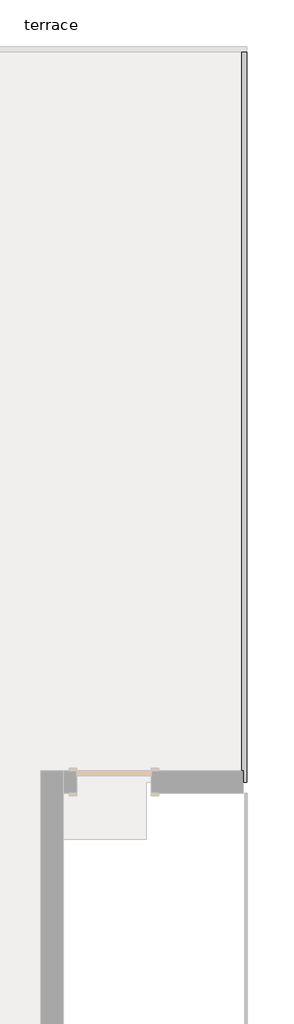
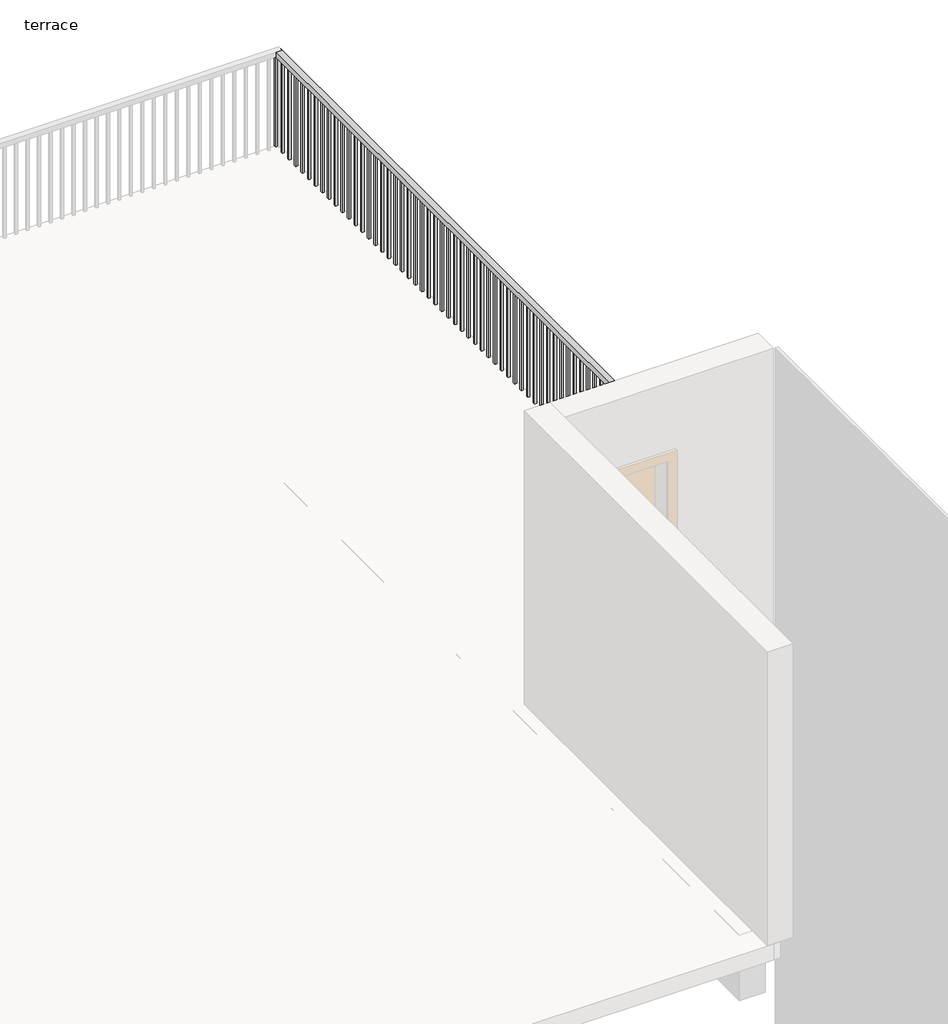
# One storey, part 6 of 6: 1 railing.
"""IFC4 building model written with IfcOpenShell, lengths in millimetres."""

from ifc_helpers import new_model, si_unit, frame, origin, place, context, project, spatial, polyline, outline, extrude, element, save

model = new_model("IFC4")

# Units and contexts
model_context = context("Model", 3, world=origin())
ifc_project = project(units=[si_unit("LENGTHUNIT", "METRE", prefix="MILLI")], contexts=[model_context])

# Site, building, storey
site = spatial("IfcSite", under=ifc_project)
building = spatial("IfcBuilding", under=site)
storey = spatial("IfcBuildingStorey", under=building, Name="terrace", Elevation=7010.4)

# Railing
placement = place(None, origin())
element("IfcRailing", 1, ObjectType="Handrail - Rectangular", at=placement, inside=storey, context=model_context, shape_type="SweptSolid", body=[
    extrude(outline(polyline([(-2647.3594779, -998.5064015), (-2698.1594779, -998.5064015), (-2698.1594779, 6526.2435985), (-2647.3594779, 6526.2435985), (-2647.3594779, -998.5064015)])), frame((0.0, 0.0, 7874.0), z_axis=(0.0, 0.0, 1.0), x_axis=(1.0, 0.0, 0.0)), (0.0, 0.0, 1.0), 50.8),
    extrude(outline(polyline([(-2663.2344779, 6510.3685985), (-2682.2844779, 6510.3685985), (-2682.2844779, 6529.4185985), (-2663.2344779, 6529.4185985), (-2663.2344779, 6510.3685985)])), frame((0.0, 0.0, 7010.4), z_axis=(0.0, 0.0, 1.0), x_axis=(1.0, 0.0, 0.0)), (0.0, 0.0, 1.0), 863.6),
    extrude(outline(polyline([(-2663.2344779, 6408.7685985), (-2682.2844779, 6408.7685985), (-2682.2844779, 6427.8185985), (-2663.2344779, 6427.8185985), (-2663.2344779, 6408.7685985)])), frame((0.0, 0.0, 7010.4), z_axis=(0.0, 0.0, 1.0), x_axis=(1.0, 0.0, 0.0)), (0.0, 0.0, 1.0), 863.6),
    extrude(outline(polyline([(-2663.2344779, 6307.1685985), (-2682.2844779, 6307.1685985), (-2682.2844779, 6326.2185985), (-2663.2344779, 6326.2185985), (-2663.2344779, 6307.1685985)])), frame((0.0, 0.0, 7010.4), z_axis=(0.0, 0.0, 1.0), x_axis=(1.0, 0.0, 0.0)), (0.0, 0.0, 1.0), 863.6),
    extrude(outline(polyline([(-2663.2344779, 6205.5685985), (-2682.2844779, 6205.5685985), (-2682.2844779, 6224.6185985), (-2663.2344779, 6224.6185985), (-2663.2344779, 6205.5685985)])), frame((0.0, 0.0, 7010.4), z_axis=(0.0, 0.0, 1.0), x_axis=(1.0, 0.0, 0.0)), (0.0, 0.0, 1.0), 863.6),
    extrude(outline(polyline([(-2663.2344779, 6103.9685985), (-2682.2844779, 6103.9685985), (-2682.2844779, 6123.0185985), (-2663.2344779, 6123.0185985), (-2663.2344779, 6103.9685985)])), frame((0.0, 0.0, 7010.4), z_axis=(0.0, 0.0, 1.0), x_axis=(1.0, 0.0, 0.0)), (0.0, 0.0, 1.0), 863.6),
    extrude(outline(polyline([(-2663.2344779, 6002.3685985), (-2682.2844779, 6002.3685985), (-2682.2844779, 6021.4185985), (-2663.2344779, 6021.4185985), (-2663.2344779, 6002.3685985)])), frame((0.0, 0.0, 7010.4), z_axis=(0.0, 0.0, 1.0), x_axis=(1.0, 0.0, 0.0)), (0.0, 0.0, 1.0), 863.6),
    extrude(outline(polyline([(-2663.2344779, 5900.7685985), (-2682.2844779, 5900.7685985), (-2682.2844779, 5919.8185985), (-2663.2344779, 5919.8185985), (-2663.2344779, 5900.7685985)])), frame((0.0, 0.0, 7010.4), z_axis=(0.0, 0.0, 1.0), x_axis=(1.0, 0.0, 0.0)), (0.0, 0.0, 1.0), 863.6),
    extrude(outline(polyline([(-2663.2344779, 5799.1685985), (-2682.2844779, 5799.1685985), (-2682.2844779, 5818.2185985), (-2663.2344779, 5818.2185985), (-2663.2344779, 5799.1685985)])), frame((0.0, 0.0, 7010.4), z_axis=(0.0, 0.0, 1.0), x_axis=(1.0, 0.0, 0.0)), (0.0, 0.0, 1.0), 863.6),
    extrude(outline(polyline([(-2663.2344779, 5697.5685985), (-2682.2844779, 5697.5685985), (-2682.2844779, 5716.6185985), (-2663.2344779, 5716.6185985), (-2663.2344779, 5697.5685985)])), frame((0.0, 0.0, 7010.4), z_axis=(0.0, 0.0, 1.0), x_axis=(1.0, 0.0, 0.0)), (0.0, 0.0, 1.0), 863.6),
    extrude(outline(polyline([(-2663.2344779, 5595.9685985), (-2682.2844779, 5595.9685985), (-2682.2844779, 5615.0185985), (-2663.2344779, 5615.0185985), (-2663.2344779, 5595.9685985)])), frame((0.0, 0.0, 7010.4), z_axis=(0.0, 0.0, 1.0), x_axis=(1.0, 0.0, 0.0)), (0.0, 0.0, 1.0), 863.6),
    extrude(outline(polyline([(-2663.2344779, 5494.3685985), (-2682.2844779, 5494.3685985), (-2682.2844779, 5513.4185985), (-2663.2344779, 5513.4185985), (-2663.2344779, 5494.3685985)])), frame((0.0, 0.0, 7010.4), z_axis=(0.0, 0.0, 1.0), x_axis=(1.0, 0.0, 0.0)), (0.0, 0.0, 1.0), 863.6),
    extrude(outline(polyline([(-2663.2344779, 5392.7685985), (-2682.2844779, 5392.7685985), (-2682.2844779, 5411.8185985), (-2663.2344779, 5411.8185985), (-2663.2344779, 5392.7685985)])), frame((0.0, 0.0, 7010.4), z_axis=(0.0, 0.0, 1.0), x_axis=(1.0, 0.0, 0.0)), (0.0, 0.0, 1.0), 863.6),
    extrude(outline(polyline([(-2663.2344779, 5291.1685985), (-2682.2844779, 5291.1685985), (-2682.2844779, 5310.2185985), (-2663.2344779, 5310.2185985), (-2663.2344779, 5291.1685985)])), frame((0.0, 0.0, 7010.4), z_axis=(0.0, 0.0, 1.0), x_axis=(1.0, 0.0, 0.0)), (0.0, 0.0, 1.0), 863.6),
    extrude(outline(polyline([(-2663.2344779, 5189.5685985), (-2682.2844779, 5189.5685985), (-2682.2844779, 5208.6185985), (-2663.2344779, 5208.6185985), (-2663.2344779, 5189.5685985)])), frame((0.0, 0.0, 7010.4), z_axis=(0.0, 0.0, 1.0), x_axis=(1.0, 0.0, 0.0)), (0.0, 0.0, 1.0), 863.6),
    extrude(outline(polyline([(-2663.2344779, 5087.9685985), (-2682.2844779, 5087.9685985), (-2682.2844779, 5107.0185985), (-2663.2344779, 5107.0185985), (-2663.2344779, 5087.9685985)])), frame((0.0, 0.0, 7010.4), z_axis=(0.0, 0.0, 1.0), x_axis=(1.0, 0.0, 0.0)), (0.0, 0.0, 1.0), 863.6),
    extrude(outline(polyline([(-2663.2344779, 4986.3685985), (-2682.2844779, 4986.3685985), (-2682.2844779, 5005.4185985), (-2663.2344779, 5005.4185985), (-2663.2344779, 4986.3685985)])), frame((0.0, 0.0, 7010.4), z_axis=(0.0, 0.0, 1.0), x_axis=(1.0, 0.0, 0.0)), (0.0, 0.0, 1.0), 863.6),
    extrude(outline(polyline([(-2663.2344779, 4884.7685985), (-2682.2844779, 4884.7685985), (-2682.2844779, 4903.8185985), (-2663.2344779, 4903.8185985), (-2663.2344779, 4884.7685985)])), frame((0.0, 0.0, 7010.4), z_axis=(0.0, 0.0, 1.0), x_axis=(1.0, 0.0, 0.0)), (0.0, 0.0, 1.0), 863.6),
    extrude(outline(polyline([(-2663.2344779, 4783.1685985), (-2682.2844779, 4783.1685985), (-2682.2844779, 4802.2185985), (-2663.2344779, 4802.2185985), (-2663.2344779, 4783.1685985)])), frame((0.0, 0.0, 7010.4), z_axis=(0.0, 0.0, 1.0), x_axis=(1.0, 0.0, 0.0)), (0.0, 0.0, 1.0), 863.6),
    extrude(outline(polyline([(-2663.2344779, 4681.5685985), (-2682.2844779, 4681.5685985), (-2682.2844779, 4700.6185985), (-2663.2344779, 4700.6185985), (-2663.2344779, 4681.5685985)])), frame((0.0, 0.0, 7010.4), z_axis=(0.0, 0.0, 1.0), x_axis=(1.0, 0.0, 0.0)), (0.0, 0.0, 1.0), 863.6),
    extrude(outline(polyline([(-2663.2344779, 4579.9685985), (-2682.2844779, 4579.9685985), (-2682.2844779, 4599.0185985), (-2663.2344779, 4599.0185985), (-2663.2344779, 4579.9685985)])), frame((0.0, 0.0, 7010.4), z_axis=(0.0, 0.0, 1.0), x_axis=(1.0, 0.0, 0.0)), (0.0, 0.0, 1.0), 863.6),
    extrude(outline(polyline([(-2663.2344779, 4478.3685985), (-2682.2844779, 4478.3685985), (-2682.2844779, 4497.4185985), (-2663.2344779, 4497.4185985), (-2663.2344779, 4478.3685985)])), frame((0.0, 0.0, 7010.4), z_axis=(0.0, 0.0, 1.0), x_axis=(1.0, 0.0, 0.0)), (0.0, 0.0, 1.0), 863.6),
    extrude(outline(polyline([(-2663.2344779, 4376.7685985), (-2682.2844779, 4376.7685985), (-2682.2844779, 4395.8185985), (-2663.2344779, 4395.8185985), (-2663.2344779, 4376.7685985)])), frame((0.0, 0.0, 7010.4), z_axis=(0.0, 0.0, 1.0), x_axis=(1.0, 0.0, 0.0)), (0.0, 0.0, 1.0), 863.6),
    extrude(outline(polyline([(-2663.2344779, 4275.1685985), (-2682.2844779, 4275.1685985), (-2682.2844779, 4294.2185985), (-2663.2344779, 4294.2185985), (-2663.2344779, 4275.1685985)])), frame((0.0, 0.0, 7010.4), z_axis=(0.0, 0.0, 1.0), x_axis=(1.0, 0.0, 0.0)), (0.0, 0.0, 1.0), 863.6),
    extrude(outline(polyline([(-2663.2344779, 4173.5685985), (-2682.2844779, 4173.5685985), (-2682.2844779, 4192.6185985), (-2663.2344779, 4192.6185985), (-2663.2344779, 4173.5685985)])), frame((0.0, 0.0, 7010.4), z_axis=(0.0, 0.0, 1.0), x_axis=(1.0, 0.0, 0.0)), (0.0, 0.0, 1.0), 863.6),
    extrude(outline(polyline([(-2663.2344779, 4071.9685985), (-2682.2844779, 4071.9685985), (-2682.2844779, 4091.0185985), (-2663.2344779, 4091.0185985), (-2663.2344779, 4071.9685985)])), frame((0.0, 0.0, 7010.4), z_axis=(0.0, 0.0, 1.0), x_axis=(1.0, 0.0, 0.0)), (0.0, 0.0, 1.0), 863.6),
    extrude(outline(polyline([(-2663.2344779, 3970.3685985), (-2682.2844779, 3970.3685985), (-2682.2844779, 3989.4185985), (-2663.2344779, 3989.4185985), (-2663.2344779, 3970.3685985)])), frame((0.0, 0.0, 7010.4), z_axis=(0.0, 0.0, 1.0), x_axis=(1.0, 0.0, 0.0)), (0.0, 0.0, 1.0), 863.6),
    extrude(outline(polyline([(-2663.2344779, 3868.7685985), (-2682.2844779, 3868.7685985), (-2682.2844779, 3887.8185985), (-2663.2344779, 3887.8185985), (-2663.2344779, 3868.7685985)])), frame((0.0, 0.0, 7010.4), z_axis=(0.0, 0.0, 1.0), x_axis=(1.0, 0.0, 0.0)), (0.0, 0.0, 1.0), 863.6),
    extrude(outline(polyline([(-2663.2344779, 3767.1685985), (-2682.2844779, 3767.1685985), (-2682.2844779, 3786.2185985), (-2663.2344779, 3786.2185985), (-2663.2344779, 3767.1685985)])), frame((0.0, 0.0, 7010.4), z_axis=(0.0, 0.0, 1.0), x_axis=(1.0, 0.0, 0.0)), (0.0, 0.0, 1.0), 863.6),
    extrude(outline(polyline([(-2663.2344779, 3665.5685985), (-2682.2844779, 3665.5685985), (-2682.2844779, 3684.6185985), (-2663.2344779, 3684.6185985), (-2663.2344779, 3665.5685985)])), frame((0.0, 0.0, 7010.4), z_axis=(0.0, 0.0, 1.0), x_axis=(1.0, 0.0, 0.0)), (0.0, 0.0, 1.0), 863.6),
    extrude(outline(polyline([(-2663.2344779, 3563.9685985), (-2682.2844779, 3563.9685985), (-2682.2844779, 3583.0185985), (-2663.2344779, 3583.0185985), (-2663.2344779, 3563.9685985)])), frame((0.0, 0.0, 7010.4), z_axis=(0.0, 0.0, 1.0), x_axis=(1.0, 0.0, 0.0)), (0.0, 0.0, 1.0), 863.6),
    extrude(outline(polyline([(-2663.2344779, 3462.3685985), (-2682.2844779, 3462.3685985), (-2682.2844779, 3481.4185985), (-2663.2344779, 3481.4185985), (-2663.2344779, 3462.3685985)])), frame((0.0, 0.0, 7010.4), z_axis=(0.0, 0.0, 1.0), x_axis=(1.0, 0.0, 0.0)), (0.0, 0.0, 1.0), 863.6),
    extrude(outline(polyline([(-2663.2344779, 3360.7685985), (-2682.2844779, 3360.7685985), (-2682.2844779, 3379.8185985), (-2663.2344779, 3379.8185985), (-2663.2344779, 3360.7685985)])), frame((0.0, 0.0, 7010.4), z_axis=(0.0, 0.0, 1.0), x_axis=(1.0, 0.0, 0.0)), (0.0, 0.0, 1.0), 863.6),
    extrude(outline(polyline([(-2663.2344779, 3259.1685985), (-2682.2844779, 3259.1685985), (-2682.2844779, 3278.2185985), (-2663.2344779, 3278.2185985), (-2663.2344779, 3259.1685985)])), frame((0.0, 0.0, 7010.4), z_axis=(0.0, 0.0, 1.0), x_axis=(1.0, 0.0, 0.0)), (0.0, 0.0, 1.0), 863.6),
    extrude(outline(polyline([(-2663.2344779, 3157.5685985), (-2682.2844779, 3157.5685985), (-2682.2844779, 3176.6185985), (-2663.2344779, 3176.6185985), (-2663.2344779, 3157.5685985)])), frame((0.0, 0.0, 7010.4), z_axis=(0.0, 0.0, 1.0), x_axis=(1.0, 0.0, 0.0)), (0.0, 0.0, 1.0), 863.6),
    extrude(outline(polyline([(-2663.2344779, 3055.9685985), (-2682.2844779, 3055.9685985), (-2682.2844779, 3075.0185985), (-2663.2344779, 3075.0185985), (-2663.2344779, 3055.9685985)])), frame((0.0, 0.0, 7010.4), z_axis=(0.0, 0.0, 1.0), x_axis=(1.0, 0.0, 0.0)), (0.0, 0.0, 1.0), 863.6),
    extrude(outline(polyline([(-2663.2344779, 2954.3685985), (-2682.2844779, 2954.3685985), (-2682.2844779, 2973.4185985), (-2663.2344779, 2973.4185985), (-2663.2344779, 2954.3685985)])), frame((0.0, 0.0, 7010.4), z_axis=(0.0, 0.0, 1.0), x_axis=(1.0, 0.0, 0.0)), (0.0, 0.0, 1.0), 863.6),
    extrude(outline(polyline([(-2663.2344779, 2852.7685985), (-2682.2844779, 2852.7685985), (-2682.2844779, 2871.8185985), (-2663.2344779, 2871.8185985), (-2663.2344779, 2852.7685985)])), frame((0.0, 0.0, 7010.4), z_axis=(0.0, 0.0, 1.0), x_axis=(1.0, 0.0, 0.0)), (0.0, 0.0, 1.0), 863.6),
    extrude(outline(polyline([(-2663.2344779, 2751.1685985), (-2682.2844779, 2751.1685985), (-2682.2844779, 2770.2185985), (-2663.2344779, 2770.2185985), (-2663.2344779, 2751.1685985)])), frame((0.0, 0.0, 7010.4), z_axis=(0.0, 0.0, 1.0), x_axis=(1.0, 0.0, 0.0)), (0.0, 0.0, 1.0), 863.6),
    extrude(outline(polyline([(-2663.2344779, 2649.5685985), (-2682.2844779, 2649.5685985), (-2682.2844779, 2668.6185985), (-2663.2344779, 2668.6185985), (-2663.2344779, 2649.5685985)])), frame((0.0, 0.0, 7010.4), z_axis=(0.0, 0.0, 1.0), x_axis=(1.0, 0.0, 0.0)), (0.0, 0.0, 1.0), 863.6),
    extrude(outline(polyline([(-2663.2344779, 2547.9685985), (-2682.2844779, 2547.9685985), (-2682.2844779, 2567.0185985), (-2663.2344779, 2567.0185985), (-2663.2344779, 2547.9685985)])), frame((0.0, 0.0, 7010.4), z_axis=(0.0, 0.0, 1.0), x_axis=(1.0, 0.0, 0.0)), (0.0, 0.0, 1.0), 863.6),
    extrude(outline(polyline([(-2663.2344779, 2446.3685985), (-2682.2844779, 2446.3685985), (-2682.2844779, 2465.4185985), (-2663.2344779, 2465.4185985), (-2663.2344779, 2446.3685985)])), frame((0.0, 0.0, 7010.4), z_axis=(0.0, 0.0, 1.0), x_axis=(1.0, 0.0, 0.0)), (0.0, 0.0, 1.0), 863.6),
    extrude(outline(polyline([(-2663.2344779, 2344.7685985), (-2682.2844779, 2344.7685985), (-2682.2844779, 2363.8185985), (-2663.2344779, 2363.8185985), (-2663.2344779, 2344.7685985)])), frame((0.0, 0.0, 7010.4), z_axis=(0.0, 0.0, 1.0), x_axis=(1.0, 0.0, 0.0)), (0.0, 0.0, 1.0), 863.6),
    extrude(outline(polyline([(-2663.2344779, 2243.1685985), (-2682.2844779, 2243.1685985), (-2682.2844779, 2262.2185985), (-2663.2344779, 2262.2185985), (-2663.2344779, 2243.1685985)])), frame((0.0, 0.0, 7010.4), z_axis=(0.0, 0.0, 1.0), x_axis=(1.0, 0.0, 0.0)), (0.0, 0.0, 1.0), 863.6),
    extrude(outline(polyline([(-2663.2344779, 2141.5685985), (-2682.2844779, 2141.5685985), (-2682.2844779, 2160.6185985), (-2663.2344779, 2160.6185985), (-2663.2344779, 2141.5685985)])), frame((0.0, 0.0, 7010.4), z_axis=(0.0, 0.0, 1.0), x_axis=(1.0, 0.0, 0.0)), (0.0, 0.0, 1.0), 863.6),
    extrude(outline(polyline([(-2663.2344779, 2039.9685985), (-2682.2844779, 2039.9685985), (-2682.2844779, 2059.0185985), (-2663.2344779, 2059.0185985), (-2663.2344779, 2039.9685985)])), frame((0.0, 0.0, 7010.4), z_axis=(0.0, 0.0, 1.0), x_axis=(1.0, 0.0, 0.0)), (0.0, 0.0, 1.0), 863.6),
    extrude(outline(polyline([(-2663.2344779, 1938.3685985), (-2682.2844779, 1938.3685985), (-2682.2844779, 1957.4185985), (-2663.2344779, 1957.4185985), (-2663.2344779, 1938.3685985)])), frame((0.0, 0.0, 7010.4), z_axis=(0.0, 0.0, 1.0), x_axis=(1.0, 0.0, 0.0)), (0.0, 0.0, 1.0), 863.6),
    extrude(outline(polyline([(-2663.2344779, 1836.7685985), (-2682.2844779, 1836.7685985), (-2682.2844779, 1855.8185985), (-2663.2344779, 1855.8185985), (-2663.2344779, 1836.7685985)])), frame((0.0, 0.0, 7010.4), z_axis=(0.0, 0.0, 1.0), x_axis=(1.0, 0.0, 0.0)), (0.0, 0.0, 1.0), 863.6),
    extrude(outline(polyline([(-2663.2344779, 1735.1685985), (-2682.2844779, 1735.1685985), (-2682.2844779, 1754.2185985), (-2663.2344779, 1754.2185985), (-2663.2344779, 1735.1685985)])), frame((0.0, 0.0, 7010.4), z_axis=(0.0, 0.0, 1.0), x_axis=(1.0, 0.0, 0.0)), (0.0, 0.0, 1.0), 863.6),
    extrude(outline(polyline([(-2663.2344779, 1633.5685985), (-2682.2844779, 1633.5685985), (-2682.2844779, 1652.6185985), (-2663.2344779, 1652.6185985), (-2663.2344779, 1633.5685985)])), frame((0.0, 0.0, 7010.4), z_axis=(0.0, 0.0, 1.0), x_axis=(1.0, 0.0, 0.0)), (0.0, 0.0, 1.0), 863.6),
    extrude(outline(polyline([(-2663.2344779, 1531.9685985), (-2682.2844779, 1531.9685985), (-2682.2844779, 1551.0185985), (-2663.2344779, 1551.0185985), (-2663.2344779, 1531.9685985)])), frame((0.0, 0.0, 7010.4), z_axis=(0.0, 0.0, 1.0), x_axis=(1.0, 0.0, 0.0)), (0.0, 0.0, 1.0), 863.6),
    extrude(outline(polyline([(-2663.2344779, 1430.3685985), (-2682.2844779, 1430.3685985), (-2682.2844779, 1449.4185985), (-2663.2344779, 1449.4185985), (-2663.2344779, 1430.3685985)])), frame((0.0, 0.0, 7010.4), z_axis=(0.0, 0.0, 1.0), x_axis=(1.0, 0.0, 0.0)), (0.0, 0.0, 1.0), 863.6),
    extrude(outline(polyline([(-2663.2344779, 1328.7685985), (-2682.2844779, 1328.7685985), (-2682.2844779, 1347.8185985), (-2663.2344779, 1347.8185985), (-2663.2344779, 1328.7685985)])), frame((0.0, 0.0, 7010.4), z_axis=(0.0, 0.0, 1.0), x_axis=(1.0, 0.0, 0.0)), (0.0, 0.0, 1.0), 863.6),
    extrude(outline(polyline([(-2663.2344779, 1227.1685985), (-2682.2844779, 1227.1685985), (-2682.2844779, 1246.2185985), (-2663.2344779, 1246.2185985), (-2663.2344779, 1227.1685985)])), frame((0.0, 0.0, 7010.4), z_axis=(0.0, 0.0, 1.0), x_axis=(1.0, 0.0, 0.0)), (0.0, 0.0, 1.0), 863.6),
    extrude(outline(polyline([(-2663.2344779, 1125.5685985), (-2682.2844779, 1125.5685985), (-2682.2844779, 1144.6185985), (-2663.2344779, 1144.6185985), (-2663.2344779, 1125.5685985)])), frame((0.0, 0.0, 7010.4), z_axis=(0.0, 0.0, 1.0), x_axis=(1.0, 0.0, 0.0)), (0.0, 0.0, 1.0), 863.6),
    extrude(outline(polyline([(-2663.2344779, 1023.9685985), (-2682.2844779, 1023.9685985), (-2682.2844779, 1043.0185985), (-2663.2344779, 1043.0185985), (-2663.2344779, 1023.9685985)])), frame((0.0, 0.0, 7010.4), z_axis=(0.0, 0.0, 1.0), x_axis=(1.0, 0.0, 0.0)), (0.0, 0.0, 1.0), 863.6),
    extrude(outline(polyline([(-2663.2344779, 922.3685985), (-2682.2844779, 922.3685985), (-2682.2844779, 941.4185985), (-2663.2344779, 941.4185985), (-2663.2344779, 922.3685985)])), frame((0.0, 0.0, 7010.4), z_axis=(0.0, 0.0, 1.0), x_axis=(1.0, 0.0, 0.0)), (0.0, 0.0, 1.0), 863.6),
    extrude(outline(polyline([(-2663.2344779, 820.7685985), (-2682.2844779, 820.7685985), (-2682.2844779, 839.8185985), (-2663.2344779, 839.8185985), (-2663.2344779, 820.7685985)])), frame((0.0, 0.0, 7010.4), z_axis=(0.0, 0.0, 1.0), x_axis=(1.0, 0.0, 0.0)), (0.0, 0.0, 1.0), 863.6),
    extrude(outline(polyline([(-2663.2344779, 719.1685985), (-2682.2844779, 719.1685985), (-2682.2844779, 738.2185985), (-2663.2344779, 738.2185985), (-2663.2344779, 719.1685985)])), frame((0.0, 0.0, 7010.4), z_axis=(0.0, 0.0, 1.0), x_axis=(1.0, 0.0, 0.0)), (0.0, 0.0, 1.0), 863.6),
    extrude(outline(polyline([(-2663.2344779, 617.5685985), (-2682.2844779, 617.5685985), (-2682.2844779, 636.6185985), (-2663.2344779, 636.6185985), (-2663.2344779, 617.5685985)])), frame((0.0, 0.0, 7010.4), z_axis=(0.0, 0.0, 1.0), x_axis=(1.0, 0.0, 0.0)), (0.0, 0.0, 1.0), 863.6),
    extrude(outline(polyline([(-2663.2344779, 515.9685985), (-2682.2844779, 515.9685985), (-2682.2844779, 535.0185985), (-2663.2344779, 535.0185985), (-2663.2344779, 515.9685985)])), frame((0.0, 0.0, 7010.4), z_axis=(0.0, 0.0, 1.0), x_axis=(1.0, 0.0, 0.0)), (0.0, 0.0, 1.0), 863.6),
    extrude(outline(polyline([(-2663.2344779, 414.3685985), (-2682.2844779, 414.3685985), (-2682.2844779, 433.4185985), (-2663.2344779, 433.4185985), (-2663.2344779, 414.3685985)])), frame((0.0, 0.0, 7010.4), z_axis=(0.0, 0.0, 1.0), x_axis=(1.0, 0.0, 0.0)), (0.0, 0.0, 1.0), 863.6),
    extrude(outline(polyline([(-2663.2344779, 312.7685985), (-2682.2844779, 312.7685985), (-2682.2844779, 331.8185985), (-2663.2344779, 331.8185985), (-2663.2344779, 312.7685985)])), frame((0.0, 0.0, 7010.4), z_axis=(0.0, 0.0, 1.0), x_axis=(1.0, 0.0, 0.0)), (0.0, 0.0, 1.0), 863.6),
    extrude(outline(polyline([(-2663.2344779, 211.1685985), (-2682.2844779, 211.1685985), (-2682.2844779, 230.2185985), (-2663.2344779, 230.2185985), (-2663.2344779, 211.1685985)])), frame((0.0, 0.0, 7010.4), z_axis=(0.0, 0.0, 1.0), x_axis=(1.0, 0.0, 0.0)), (0.0, 0.0, 1.0), 863.6),
    extrude(outline(polyline([(-2663.2344779, 109.5685985), (-2682.2844779, 109.5685985), (-2682.2844779, 128.6185985), (-2663.2344779, 128.6185985), (-2663.2344779, 109.5685985)])), frame((0.0, 0.0, 7010.4), z_axis=(0.0, 0.0, 1.0), x_axis=(1.0, 0.0, 0.0)), (0.0, 0.0, 1.0), 863.6),
    extrude(outline(polyline([(-2663.2344779, 7.9685985), (-2682.2844779, 7.9685985), (-2682.2844779, 27.0185985), (-2663.2344779, 27.0185985), (-2663.2344779, 7.9685985)])), frame((0.0, 0.0, 7010.4), z_axis=(0.0, 0.0, 1.0), x_axis=(1.0, 0.0, 0.0)), (0.0, 0.0, 1.0), 863.6),
    extrude(outline(polyline([(-2663.2344779, -93.6314015), (-2682.2844779, -93.6314015), (-2682.2844779, -74.5814015), (-2663.2344779, -74.5814015), (-2663.2344779, -93.6314015)])), frame((0.0, 0.0, 7010.4), z_axis=(0.0, 0.0, 1.0), x_axis=(1.0, 0.0, 0.0)), (0.0, 0.0, 1.0), 863.6),
    extrude(outline(polyline([(-2663.2344779, -195.2314015), (-2682.2844779, -195.2314015), (-2682.2844779, -176.1814015), (-2663.2344779, -176.1814015), (-2663.2344779, -195.2314015)])), frame((0.0, 0.0, 7010.4), z_axis=(0.0, 0.0, 1.0), x_axis=(1.0, 0.0, 0.0)), (0.0, 0.0, 1.0), 863.6),
    extrude(outline(polyline([(-2663.2344779, -296.8314015), (-2682.2844779, -296.8314015), (-2682.2844779, -277.7814015), (-2663.2344779, -277.7814015), (-2663.2344779, -296.8314015)])), frame((0.0, 0.0, 7010.4), z_axis=(0.0, 0.0, 1.0), x_axis=(1.0, 0.0, 0.0)), (0.0, 0.0, 1.0), 863.6),
    extrude(outline(polyline([(-2663.2344779, -398.4314015), (-2682.2844779, -398.4314015), (-2682.2844779, -379.3814015), (-2663.2344779, -379.3814015), (-2663.2344779, -398.4314015)])), frame((0.0, 0.0, 7010.4), z_axis=(0.0, 0.0, 1.0), x_axis=(1.0, 0.0, 0.0)), (0.0, 0.0, 1.0), 863.6),
    extrude(outline(polyline([(-2663.2344779, -500.0314015), (-2682.2844779, -500.0314015), (-2682.2844779, -480.9814015), (-2663.2344779, -480.9814015), (-2663.2344779, -500.0314015)])), frame((0.0, 0.0, 7010.4), z_axis=(0.0, 0.0, 1.0), x_axis=(1.0, 0.0, 0.0)), (0.0, 0.0, 1.0), 863.6),
    extrude(outline(polyline([(-2663.2344779, -601.6314015), (-2682.2844779, -601.6314015), (-2682.2844779, -582.5814015), (-2663.2344779, -582.5814015), (-2663.2344779, -601.6314015)])), frame((0.0, 0.0, 7010.4), z_axis=(0.0, 0.0, 1.0), x_axis=(1.0, 0.0, 0.0)), (0.0, 0.0, 1.0), 863.6),
    extrude(outline(polyline([(-2663.2344779, -703.2314015), (-2682.2844779, -703.2314015), (-2682.2844779, -684.1814015), (-2663.2344779, -684.1814015), (-2663.2344779, -703.2314015)])), frame((0.0, 0.0, 7010.4), z_axis=(0.0, 0.0, 1.0), x_axis=(1.0, 0.0, 0.0)), (0.0, 0.0, 1.0), 863.6),
    extrude(outline(polyline([(-2663.2344779, -804.8314015), (-2682.2844779, -804.8314015), (-2682.2844779, -785.7814015), (-2663.2344779, -785.7814015), (-2663.2344779, -804.8314015)])), frame((0.0, 0.0, 7010.4), z_axis=(0.0, 0.0, 1.0), x_axis=(1.0, 0.0, 0.0)), (0.0, 0.0, 1.0), 863.6),
    extrude(outline(polyline([(-2663.2344779, -906.4314015), (-2682.2844779, -906.4314015), (-2682.2844779, -887.3814015), (-2663.2344779, -887.3814015), (-2663.2344779, -906.4314015)])), frame((0.0, 0.0, 7010.4), z_axis=(0.0, 0.0, 1.0), x_axis=(1.0, 0.0, 0.0)), (0.0, 0.0, 1.0), 863.6),
    extrude(outline(polyline([(-2663.2344779, 6507.1935985), (-2682.2844779, 6507.1935985), (-2682.2844779, 6526.2435985), (-2663.2344779, 6526.2435985), (-2663.2344779, 6507.1935985)])), frame((0.0, 0.0, 7010.4), z_axis=(0.0, 0.0, 1.0), x_axis=(1.0, 0.0, 0.0)), (0.0, 0.0, 1.0), 863.6),
    extrude(outline(polyline([(-2663.2344779, -998.5064015), (-2682.2844779, -998.5064015), (-2682.2844779, -979.4564015), (-2663.2344779, -979.4564015), (-2663.2344779, -998.5064015)])), frame((0.0, 0.0, 7010.4), z_axis=(0.0, 0.0, 1.0), x_axis=(1.0, 0.0, 0.0)), (0.0, 0.0, 1.0), 863.6),
])

save(model, "model.ifc")

# Revit data of these elements
# Type "Handrail - Rectangular"
#   Assembly Code = "C2010400"
#   built-in parameter 1008612 = 0.0416667 (stored number, unit not read)
#   built-in parameter 1008611 = 0.0416667 (stored number, unit not read)
#   built-in parameter 1008609 = 0.333333 (stored number, unit not read)
#   built-in parameter 1008604 = 0.166667 (stored number, unit not read)
#   built-in parameter 1008603 = 0.166667 (stored number, unit not read)
#   Railing Height = 3' - 0"
#   built-in parameter 1008630 = 2
#   built-in parameter 1008610 = 2
#   built-in parameter 1008618 = Baluster - Square : 3/4"
# Element 1 (IfcRailing, "Handrail - Rectangular")
#   Phase Created = New Construction
